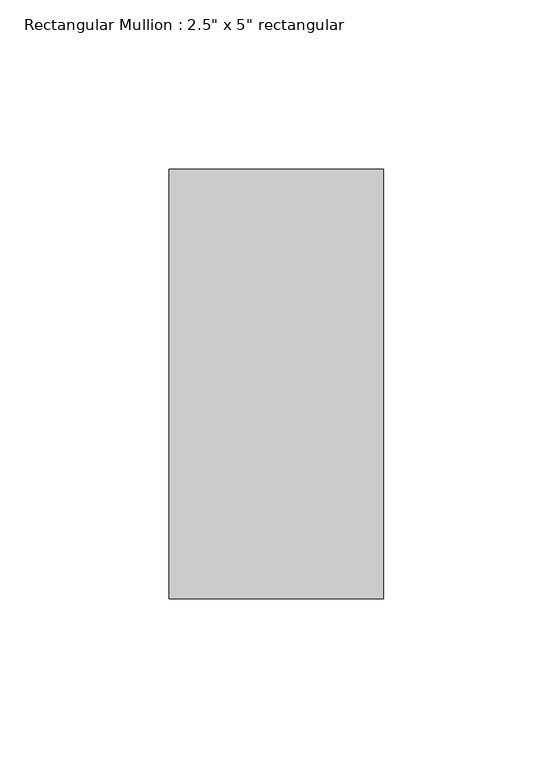
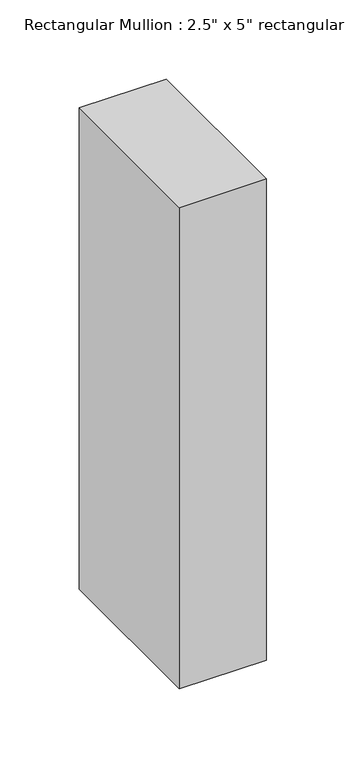
"""IFC4 building model written with IfcOpenShell, lengths in millimetres: member geometry."""

from ifc_helpers import new_model, si_unit, frame, origin, place, context, project, spatial, polyline, outline, extrude, source, transform, mapped, element, save


def member_76ae402a(model_context):
    return source(origin(), model_context, "Body", "SweptSolid", [
        extrude(outline(polyline([(31.75, 63.5), (31.75, -63.5), (-31.75, -63.5), (-31.75, 63.5), (31.75, 63.5)])), frame((0.0, 0.0, -371.5546147), z_axis=(0.0, 0.0, 1.0), x_axis=(1.0, 0.0, 0.0)), (0.0, 0.0, 1.0), 371.5546147),
    ])


if __name__ == "__main__":
    model = new_model("IFC4")
    model_context = context("Model", 3, world=origin())
    ifc_project = project(units=[si_unit("LENGTHUNIT", "METRE", prefix="MILLI")], contexts=[model_context])
    site = spatial("IfcSite", under=ifc_project)
    building = spatial("IfcBuilding", under=site)
    placement = place(None, origin())
    member_shape = member_76ae402a(model_context)
    element("IfcMember", 1, ObjectType="Rectangular Mullion : 2.5\" x 5\" rectangular", at=placement, inside=building, context=model_context, shape_type="MappedRepresentation", body=[
        mapped(member_shape, transform((0.0, 0.0, 0.0), x_axis=(1.0, 0.0, 0.0), y_axis=(0.0, 1.0, 0.0), z_axis=(0.0, 0.0, 1.0))),
    ])
    save(model, "model.ifc")

# Revit data of these elements
# Type "Rectangular Mullion : 2.5\" x 5\" rectangular"
#   built-in parameter 1007304 = 0.416667 (stored number, unit not read)
#   built-in parameter 1007301 = 0.104167 (stored number, unit not read)
#   built-in parameter 1007300 = 0.104167 (stored number, unit not read)
